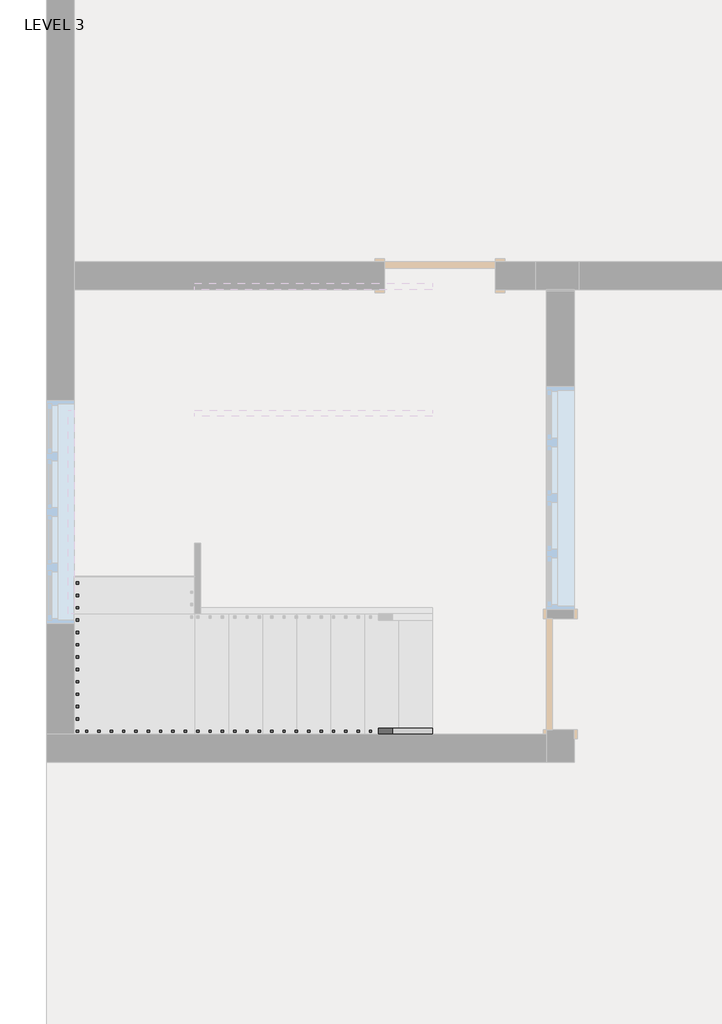
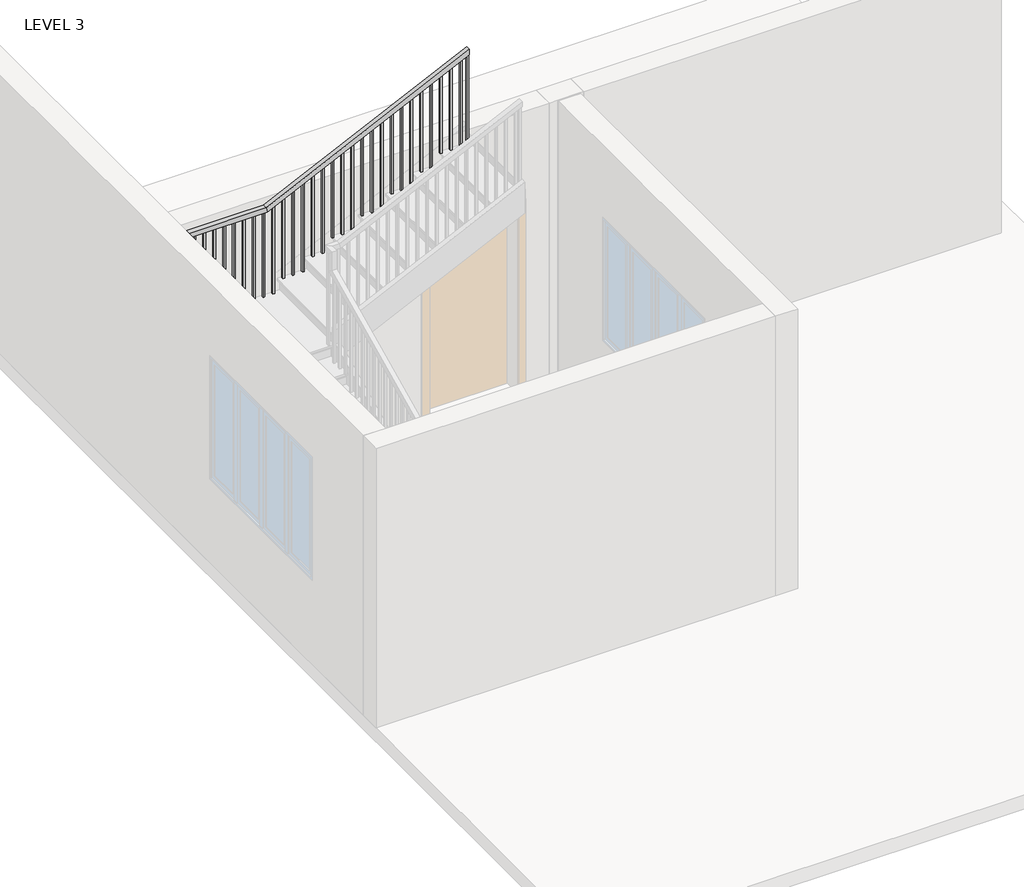
# One storey, part 2 of 3: 1 railing.
"""IFC4 building model written with IfcOpenShell, lengths in millimetres."""

from ifc_helpers import new_model, si_unit, frame, origin, place, context, project, spatial, polyline, outline, extrude, faceted_brep, element, save

model = new_model("IFC4")

# Units and contexts
model_context = context("Model", 3, world=origin())
ifc_project = project(units=[si_unit("LENGTHUNIT", "METRE", prefix="MILLI")], contexts=[model_context])

# Site, building, storey
site = spatial("IfcSite", under=ifc_project)
building = spatial("IfcBuilding", under=site)
storey = spatial("IfcBuildingStorey", under=building, Name="LEVEL 3", Elevation=6248.4)

# Railing
placement = place(None, origin())
element("IfcRailing", 1, ObjectType="Handrail - Rectangular", at=placement, inside=storey, context=model_context, shape_type="SolidModel", body=[
    faceted_brep([(-19769.8789184, -1118.4399287, 7295.3217391), (-19769.8789184, -1118.4399287, 7239.0971684), (-19769.8789184, -1067.6399287, 7239.0971684), (-19769.8789184, -1067.6399287, 7295.3217391), (-21865.3789184, -1118.4399287, 8289.2347826), (-21876.8157218, -1118.4399287, 8238.4347826), (-21876.8157218, -1067.6399287, 8238.4347826), (-21865.3789184, -1067.6399287, 8289.2347826), (-22716.2789184, -1118.4399287, 8238.4347826), (-22716.2789184, -1118.4399287, 8289.2347826), (-22716.2789184, -267.5399287, 8289.2347826), (-22716.2789184, -256.1031254, 8238.4347826), (-22665.4789184, -1067.6399287, 8238.4347826), (-22665.4789184, -256.1031254, 8238.4347826), (-22665.4789184, -1067.6399287, 8289.2347826), (-22665.4789184, -267.5399287, 8289.2347826), (-22716.2789184, 2539.1600713, 9166.0869565), (-22716.2789184, 2539.1600713, 9216.8869565), (-21865.3789184, 2539.1600713, 9216.8869565), (-21853.9421151, 2539.1600713, 9166.0869565), (-22665.4789184, 2488.3600713, 9166.0869565), (-21853.9421151, 2488.3600713, 9166.0869565), (-22665.4789184, 2488.3600713, 9216.8869565), (-21865.3789184, 2488.3600713, 9216.8869565), (-22716.2789184, 1688.2600713, 9216.8869565), (-22716.2789184, 1699.6968746, 9166.0869565), (-22665.4789184, 1699.6968746, 9166.0869565), (-22665.4789184, 1688.2600713, 9216.8869565), (-19769.8789184, 2539.1600713, 10210.8), (-19769.8789184, 2488.3600713, 10210.8), (-19769.8789184, 2488.3600713, 10154.5754292), (-19769.8789184, 2539.1600713, 10154.5754292)], [[[0, 1, 2, 3]], [[1, 0, 4, 5]], [[2, 1, 5, 6]], [[3, 2, 6, 7]], [[0, 3, 7, 4]], [[8, 9, 10, 11]], [[12, 8, 11, 13]], [[14, 12, 13, 15]], [[9, 14, 15, 10]], [[16, 17, 18, 19]], [[20, 16, 19, 21]], [[22, 20, 21, 23]], [[17, 22, 23, 18]], [[5, 4, 9, 8]], [[6, 5, 8, 12]], [[7, 6, 12, 14]], [[4, 7, 14, 9]], [[11, 10, 24, 25]], [[13, 11, 25, 26]], [[15, 13, 26, 27]], [[10, 15, 27, 24]], [[25, 24, 17, 16]], [[26, 25, 16, 20]], [[27, 26, 20, 22]], [[24, 27, 22, 17]], [[28, 29, 30, 31]], [[19, 18, 28, 31]], [[21, 19, 31, 30]], [[23, 21, 30, 29]], [[18, 23, 29, 28]]]),
    extrude(outline(polyline([(10113.9153502, -19855.6039184), (9163.8782609, -19855.6039184), (9163.8782609, -19836.5539184), (10122.9509233, -19836.5539184), (10113.9153502, -19855.6039184)])), frame((0.0, 2504.2350713, 0.0), z_axis=(0.0, 1.0, 0.0), x_axis=(0.0, 0.0, 1.0)), (0.0, 0.0, 1.0), 19.05),
    extrude(outline(polyline([(10065.7256269, -19957.2039184), (9163.8782609, -19957.2039184), (9163.8782609, -19938.1539184), (10074.7612, -19938.1539184), (10065.7256269, -19957.2039184)])), frame((0.0, 2504.2350713, 0.0), z_axis=(0.0, 1.0, 0.0), x_axis=(0.0, 0.0, 1.0)), (0.0, 0.0, 1.0), 19.05),
    extrude(outline(polyline([(10017.5359035, -20058.8039184), (9163.8782609, -20058.8039184), (9163.8782609, -20039.7539184), (10026.5714767, -20039.7539184), (10017.5359035, -20058.8039184)])), frame((0.0, 2504.2350713, 0.0), z_axis=(0.0, 1.0, 0.0), x_axis=(0.0, 0.0, 1.0)), (0.0, 0.0, 1.0), 19.05),
    extrude(outline(polyline([(9969.3461802, -20160.4039184), (9031.3565217, -20160.4039184), (9031.3565217, -20141.3539184), (9978.3817533, -20141.3539184), (9969.3461802, -20160.4039184)])), frame((0.0, 2504.2350713, 0.0), z_axis=(0.0, 1.0, 0.0), x_axis=(0.0, 0.0, 1.0)), (0.0, 0.0, 1.0), 19.05),
    extrude(outline(polyline([(9921.1564569, -20262.0039184), (9031.3565217, -20262.0039184), (9031.3565217, -20242.9539184), (9930.19203, -20242.9539184), (9921.1564569, -20262.0039184)])), frame((0.0, 2504.2350713, 0.0), z_axis=(0.0, 1.0, 0.0), x_axis=(0.0, 0.0, 1.0)), (0.0, 0.0, 1.0), 19.05),
    extrude(outline(polyline([(9872.9667336, -20363.6039184), (8898.8347826, -20363.6039184), (8898.8347826, -20344.5539184), (9882.0023067, -20344.5539184), (9872.9667336, -20363.6039184)])), frame((0.0, 2504.2350713, 0.0), z_axis=(0.0, 1.0, 0.0), x_axis=(0.0, 0.0, 1.0)), (0.0, 0.0, 1.0), 19.05),
    extrude(outline(polyline([(9824.7770103, -20465.2039184), (8898.8347826, -20465.2039184), (8898.8347826, -20446.1539184), (9833.8125834, -20446.1539184), (9824.7770103, -20465.2039184)])), frame((0.0, 2504.2350713, 0.0), z_axis=(0.0, 1.0, 0.0), x_axis=(0.0, 0.0, 1.0)), (0.0, 0.0, 1.0), 19.05),
    extrude(outline(polyline([(9776.5872869, -20566.8039184), (8898.8347826, -20566.8039184), (8898.8347826, -20547.7539184), (9785.6228601, -20547.7539184), (9776.5872869, -20566.8039184)])), frame((0.0, 2504.2350713, 0.0), z_axis=(0.0, 1.0, 0.0), x_axis=(0.0, 0.0, 1.0)), (0.0, 0.0, 1.0), 19.05),
    extrude(outline(polyline([(9728.3975636, -20668.4039184), (8766.3130435, -20668.4039184), (8766.3130435, -20649.3539184), (9737.4331367, -20649.3539184), (9728.3975636, -20668.4039184)])), frame((0.0, 2504.2350713, 0.0), z_axis=(0.0, 1.0, 0.0), x_axis=(0.0, 0.0, 1.0)), (0.0, 0.0, 1.0), 19.05),
    extrude(outline(polyline([(9680.2078403, -20770.0039184), (8766.3130435, -20770.0039184), (8766.3130435, -20750.9539184), (9689.2434134, -20750.9539184), (9680.2078403, -20770.0039184)])), frame((0.0, 2504.2350713, 0.0), z_axis=(0.0, 1.0, 0.0), x_axis=(0.0, 0.0, 1.0)), (0.0, 0.0, 1.0), 19.05),
    extrude(outline(polyline([(9632.018117, -20871.6039184), (8766.3130435, -20871.6039184), (8766.3130435, -20852.5539184), (9641.0536901, -20852.5539184), (9632.018117, -20871.6039184)])), frame((0.0, 2504.2350713, 0.0), z_axis=(0.0, 1.0, 0.0), x_axis=(0.0, 0.0, 1.0)), (0.0, 0.0, 1.0), 19.05),
    extrude(outline(polyline([(9583.8283937, -20973.2039184), (8633.7913043, -20973.2039184), (8633.7913043, -20954.1539184), (9592.8639668, -20954.1539184), (9583.8283937, -20973.2039184)])), frame((0.0, 2504.2350713, 0.0), z_axis=(0.0, 1.0, 0.0), x_axis=(0.0, 0.0, 1.0)), (0.0, 0.0, 1.0), 19.05),
    extrude(outline(polyline([(9535.6386703, -21074.8039184), (8633.7913043, -21074.8039184), (8633.7913043, -21055.7539184), (9544.6742435, -21055.7539184), (9535.6386703, -21074.8039184)])), frame((0.0, 2504.2350713, 0.0), z_axis=(0.0, 1.0, 0.0), x_axis=(0.0, 0.0, 1.0)), (0.0, 0.0, 1.0), 19.05),
    extrude(outline(polyline([(9487.448947, -21176.4039184), (8633.7913043, -21176.4039184), (8633.7913043, -21157.3539184), (9496.4845201, -21157.3539184), (9487.448947, -21176.4039184)])), frame((0.0, 2504.2350713, 0.0), z_axis=(0.0, 1.0, 0.0), x_axis=(0.0, 0.0, 1.0)), (0.0, 0.0, 1.0), 19.05),
    extrude(outline(polyline([(9439.2592237, -21278.0039184), (8501.2695652, -21278.0039184), (8501.2695652, -21258.9539184), (9448.2947968, -21258.9539184), (9439.2592237, -21278.0039184)])), frame((0.0, 2504.2350713, 0.0), z_axis=(0.0, 1.0, 0.0), x_axis=(0.0, 0.0, 1.0)), (0.0, 0.0, 1.0), 19.05),
    extrude(outline(polyline([(9391.0695004, -21379.6039184), (8501.2695652, -21379.6039184), (8501.2695652, -21360.5539184), (9400.1050735, -21360.5539184), (9391.0695004, -21379.6039184)])), frame((0.0, 2504.2350713, 0.0), z_axis=(0.0, 1.0, 0.0), x_axis=(0.0, 0.0, 1.0)), (0.0, 0.0, 1.0), 19.05),
    extrude(outline(polyline([(9342.8797771, -21481.2039184), (8368.7478261, -21481.2039184), (8368.7478261, -21462.1539184), (9351.9153502, -21462.1539184), (9342.8797771, -21481.2039184)])), frame((0.0, 2504.2350713, 0.0), z_axis=(0.0, 1.0, 0.0), x_axis=(0.0, 0.0, 1.0)), (0.0, 0.0, 1.0), 19.05),
    extrude(outline(polyline([(9294.6900537, -21582.8039184), (8368.7478261, -21582.8039184), (8368.7478261, -21563.7539184), (9303.7256269, -21563.7539184), (9294.6900537, -21582.8039184)])), frame((0.0, 2504.2350713, 0.0), z_axis=(0.0, 1.0, 0.0), x_axis=(0.0, 0.0, 1.0)), (0.0, 0.0, 1.0), 19.05),
    extrude(outline(polyline([(9246.5003304, -21684.4039184), (8368.7478261, -21684.4039184), (8368.7478261, -21665.3539184), (9255.5359035, -21665.3539184), (9246.5003304, -21684.4039184)])), frame((0.0, 2504.2350713, 0.0), z_axis=(0.0, 1.0, 0.0), x_axis=(0.0, 0.0, 1.0)), (0.0, 0.0, 1.0), 19.05),
    extrude(outline(polyline([(9198.3106071, -21786.0039184), (8236.226087, -21786.0039184), (8236.226087, -21766.9539184), (9207.3461802, -21766.9539184), (9198.3106071, -21786.0039184)])), frame((0.0, 2504.2350713, 0.0), z_axis=(0.0, 1.0, 0.0), x_axis=(0.0, 0.0, 1.0)), (0.0, 0.0, 1.0), 19.05),
    extrude(outline(polyline([(-21887.6039184, 2523.2850713), (-21868.5539184, 2523.2850713), (-21868.5539184, 2504.2350713), (-21887.6039184, 2504.2350713), (-21887.6039184, 2523.2850713)])), frame((0.0, 0.0, 8236.226087), z_axis=(0.0, 0.0, 1.0), x_axis=(1.0, 0.0, 0.0)), (0.0, 0.0, 1.0), 929.8608696),
    extrude(outline(polyline([(-21989.2039184, 2523.2850713), (-21970.1539184, 2523.2850713), (-21970.1539184, 2504.2350713), (-21989.2039184, 2504.2350713), (-21989.2039184, 2523.2850713)])), frame((0.0, 0.0, 8236.226087), z_axis=(0.0, 0.0, 1.0), x_axis=(1.0, 0.0, 0.0)), (0.0, 0.0, 1.0), 929.8608696),
    extrude(outline(polyline([(-22090.8039184, 2523.2850713), (-22071.7539184, 2523.2850713), (-22071.7539184, 2504.2350713), (-22090.8039184, 2504.2350713), (-22090.8039184, 2523.2850713)])), frame((0.0, 0.0, 8236.226087), z_axis=(0.0, 0.0, 1.0), x_axis=(1.0, 0.0, 0.0)), (0.0, 0.0, 1.0), 929.8608696),
    extrude(outline(polyline([(-22192.4039184, 2523.2850713), (-22173.3539184, 2523.2850713), (-22173.3539184, 2504.2350713), (-22192.4039184, 2504.2350713), (-22192.4039184, 2523.2850713)])), frame((0.0, 0.0, 8236.226087), z_axis=(0.0, 0.0, 1.0), x_axis=(1.0, 0.0, 0.0)), (0.0, 0.0, 1.0), 929.8608696),
    extrude(outline(polyline([(-22294.0039184, 2523.2850713), (-22274.9539184, 2523.2850713), (-22274.9539184, 2504.2350713), (-22294.0039184, 2504.2350713), (-22294.0039184, 2523.2850713)])), frame((0.0, 0.0, 8236.226087), z_axis=(0.0, 0.0, 1.0), x_axis=(1.0, 0.0, 0.0)), (0.0, 0.0, 1.0), 929.8608696),
    extrude(outline(polyline([(-22395.6039184, 2523.2850713), (-22376.5539184, 2523.2850713), (-22376.5539184, 2504.2350713), (-22395.6039184, 2504.2350713), (-22395.6039184, 2523.2850713)])), frame((0.0, 0.0, 8236.226087), z_axis=(0.0, 0.0, 1.0), x_axis=(1.0, 0.0, 0.0)), (0.0, 0.0, 1.0), 929.8608696),
    extrude(outline(polyline([(-22497.2039184, 2523.2850713), (-22478.1539184, 2523.2850713), (-22478.1539184, 2504.2350713), (-22497.2039184, 2504.2350713), (-22497.2039184, 2523.2850713)])), frame((0.0, 0.0, 8236.226087), z_axis=(0.0, 0.0, 1.0), x_axis=(1.0, 0.0, 0.0)), (0.0, 0.0, 1.0), 929.8608696),
    extrude(outline(polyline([(-22598.8039184, 2523.2850713), (-22579.7539184, 2523.2850713), (-22579.7539184, 2504.2350713), (-22598.8039184, 2504.2350713), (-22598.8039184, 2523.2850713)])), frame((0.0, 0.0, 8236.226087), z_axis=(0.0, 0.0, 1.0), x_axis=(1.0, 0.0, 0.0)), (0.0, 0.0, 1.0), 929.8608696),
    extrude(outline(polyline([(-22700.4039184, 2453.4350713), (-22700.4039184, 2472.4850713), (-22681.3539184, 2472.4850713), (-22681.3539184, 2453.4350713), (-22700.4039184, 2453.4350713)])), frame((0.0, 0.0, 8236.226087), z_axis=(0.0, 0.0, 1.0), x_axis=(1.0, 0.0, 0.0)), (0.0, 0.0, 1.0), 929.8608696),
    extrude(outline(polyline([(-22700.4039184, 2351.8350713), (-22700.4039184, 2370.8850713), (-22681.3539184, 2370.8850713), (-22681.3539184, 2351.8350713), (-22700.4039184, 2351.8350713)])), frame((0.0, 0.0, 8236.226087), z_axis=(0.0, 0.0, 1.0), x_axis=(1.0, 0.0, 0.0)), (0.0, 0.0, 1.0), 929.8608696),
    extrude(outline(polyline([(-22700.4039184, 2250.2350713), (-22700.4039184, 2269.2850713), (-22681.3539184, 2269.2850713), (-22681.3539184, 2250.2350713), (-22700.4039184, 2250.2350713)])), frame((0.0, 0.0, 8236.226087), z_axis=(0.0, 0.0, 1.0), x_axis=(1.0, 0.0, 0.0)), (0.0, 0.0, 1.0), 929.8608696),
    extrude(outline(polyline([(-22700.4039184, 2148.6350713), (-22700.4039184, 2167.6850713), (-22681.3539184, 2167.6850713), (-22681.3539184, 2148.6350713), (-22700.4039184, 2148.6350713)])), frame((0.0, 0.0, 8236.226087), z_axis=(0.0, 0.0, 1.0), x_axis=(1.0, 0.0, 0.0)), (0.0, 0.0, 1.0), 929.8608696),
    extrude(outline(polyline([(-22700.4039184, 2047.0350713), (-22700.4039184, 2066.0850713), (-22681.3539184, 2066.0850713), (-22681.3539184, 2047.0350713), (-22700.4039184, 2047.0350713)])), frame((0.0, 0.0, 8236.226087), z_axis=(0.0, 0.0, 1.0), x_axis=(1.0, 0.0, 0.0)), (0.0, 0.0, 1.0), 929.8608696),
    extrude(outline(polyline([(-22700.4039184, 1945.4350713), (-22700.4039184, 1964.4850713), (-22681.3539184, 1964.4850713), (-22681.3539184, 1945.4350713), (-22700.4039184, 1945.4350713)])), frame((0.0, 0.0, 8236.226087), z_axis=(0.0, 0.0, 1.0), x_axis=(1.0, 0.0, 0.0)), (0.0, 0.0, 1.0), 929.8608696),
    extrude(outline(polyline([(-22700.4039184, 1843.8350713), (-22700.4039184, 1862.8850713), (-22681.3539184, 1862.8850713), (-22681.3539184, 1843.8350713), (-22700.4039184, 1843.8350713)])), frame((0.0, 0.0, 8236.226087), z_axis=(0.0, 0.0, 1.0), x_axis=(1.0, 0.0, 0.0)), (0.0, 0.0, 1.0), 929.8608696),
    extrude(outline(polyline([(-22700.4039184, 1742.2350713), (-22700.4039184, 1761.2850713), (-22681.3539184, 1761.2850713), (-22681.3539184, 1742.2350713), (-22700.4039184, 1742.2350713)])), frame((0.0, 0.0, 8236.226087), z_axis=(0.0, 0.0, 1.0), x_axis=(1.0, 0.0, 0.0)), (0.0, 0.0, 1.0), 929.8608696),
    extrude(outline(polyline([(1659.6850713, 9147.1090261), (1659.6850713, 8236.226087), (1640.6350713, 8236.226087), (1640.6350713, 9138.0734529), (1659.6850713, 9147.1090261)])), frame((-22700.4039184, 0.0, 0.0), z_axis=(1.0, 0.0, 0.0), x_axis=(0.0, 1.0, 0.0)), (0.0, 0.0, 1.0), 19.05),
    extrude(outline(polyline([(1558.0850713, 9098.9193027), (1558.0850713, 8236.226087), (1539.0350713, 8236.226087), (1539.0350713, 9089.8837296), (1558.0850713, 9098.9193027)])), frame((-22700.4039184, 0.0, 0.0), z_axis=(1.0, 0.0, 0.0), x_axis=(0.0, 1.0, 0.0)), (0.0, 0.0, 1.0), 19.05),
    extrude(outline(polyline([(1456.4850713, 9050.7295794), (1456.4850713, 8103.7043478), (1437.4350713, 8103.7043478), (1437.4350713, 9041.6940063), (1456.4850713, 9050.7295794)])), frame((-22700.4039184, 0.0, 0.0), z_axis=(1.0, 0.0, 0.0), x_axis=(0.0, 1.0, 0.0)), (0.0, 0.0, 1.0), 19.05),
    extrude(outline(polyline([(1354.8850713, 9002.5398561), (1354.8850713, 8103.7043478), (1335.8350713, 8103.7043478), (1335.8350713, 8993.504283), (1354.8850713, 9002.5398561)])), frame((-22700.4039184, 0.0, 0.0), z_axis=(1.0, 0.0, 0.0), x_axis=(0.0, 1.0, 0.0)), (0.0, 0.0, 1.0), 19.05),
    extrude(outline(polyline([(1253.2850713, 8954.3501328), (1253.2850713, 7971.1826087), (1234.2350713, 7971.1826087), (1234.2350713, 8945.3145597), (1253.2850713, 8954.3501328)])), frame((-22700.4039184, 0.0, 0.0), z_axis=(1.0, 0.0, 0.0), x_axis=(0.0, 1.0, 0.0)), (0.0, 0.0, 1.0), 19.05),
    extrude(outline(polyline([(1151.6850713, 8906.1604095), (1151.6850713, 7971.1826087), (1132.6350713, 7971.1826087), (1132.6350713, 8897.1248363), (1151.6850713, 8906.1604095)])), frame((-22700.4039184, 0.0, 0.0), z_axis=(1.0, 0.0, 0.0), x_axis=(0.0, 1.0, 0.0)), (0.0, 0.0, 1.0), 19.05),
    extrude(outline(polyline([(1050.0850713, 8857.9706861), (1050.0850713, 7971.1826087), (1031.0350713, 7971.1826087), (1031.0350713, 8848.935113), (1050.0850713, 8857.9706861)])), frame((-22700.4039184, 0.0, 0.0), z_axis=(1.0, 0.0, 0.0), x_axis=(0.0, 1.0, 0.0)), (0.0, 0.0, 1.0), 19.05),
    extrude(outline(polyline([(948.4850713, 8809.7809628), (948.4850713, 7838.6608696), (929.4350713, 7838.6608696), (929.4350713, 8800.7453897), (948.4850713, 8809.7809628)])), frame((-22700.4039184, 0.0, 0.0), z_axis=(1.0, 0.0, 0.0), x_axis=(0.0, 1.0, 0.0)), (0.0, 0.0, 1.0), 19.05),
    extrude(outline(polyline([(846.8850713, 8761.5912395), (846.8850713, 7838.6608696), (827.8350713, 7838.6608696), (827.8350713, 8752.5556664), (846.8850713, 8761.5912395)])), frame((-22700.4039184, 0.0, 0.0), z_axis=(1.0, 0.0, 0.0), x_axis=(0.0, 1.0, 0.0)), (0.0, 0.0, 1.0), 19.05),
    extrude(outline(polyline([(745.2850713, 8713.4015162), (745.2850713, 7838.6608696), (726.2350713, 7838.6608696), (726.2350713, 8704.3659431), (745.2850713, 8713.4015162)])), frame((-22700.4039184, 0.0, 0.0), z_axis=(1.0, 0.0, 0.0), x_axis=(0.0, 1.0, 0.0)), (0.0, 0.0, 1.0), 19.05),
    extrude(outline(polyline([(643.6850713, 8665.2117929), (643.6850713, 7706.1391304), (624.6350713, 7706.1391304), (624.6350713, 8656.1762197), (643.6850713, 8665.2117929)])), frame((-22700.4039184, 0.0, 0.0), z_axis=(1.0, 0.0, 0.0), x_axis=(0.0, 1.0, 0.0)), (0.0, 0.0, 1.0), 19.05),
    extrude(outline(polyline([(542.0850713, 8617.0220695), (542.0850713, 7706.1391304), (523.0350713, 7706.1391304), (523.0350713, 8607.9864964), (542.0850713, 8617.0220695)])), frame((-22700.4039184, 0.0, 0.0), z_axis=(1.0, 0.0, 0.0), x_axis=(0.0, 1.0, 0.0)), (0.0, 0.0, 1.0), 19.05),
    extrude(outline(polyline([(440.4850713, 8568.8323462), (440.4850713, 7706.1391304), (421.4350713, 7706.1391304), (421.4350713, 8559.7967731), (440.4850713, 8568.8323462)])), frame((-22700.4039184, 0.0, 0.0), z_axis=(1.0, 0.0, 0.0), x_axis=(0.0, 1.0, 0.0)), (0.0, 0.0, 1.0), 19.05),
    extrude(outline(polyline([(338.8850713, 8520.6426229), (338.8850713, 7573.6173913), (319.8350713, 7573.6173913), (319.8350713, 8511.6070498), (338.8850713, 8520.6426229)])), frame((-22700.4039184, 0.0, 0.0), z_axis=(1.0, 0.0, 0.0), x_axis=(0.0, 1.0, 0.0)), (0.0, 0.0, 1.0), 19.05),
    extrude(outline(polyline([(237.2850713, 8472.4528996), (237.2850713, 7573.6173913), (218.2350713, 7573.6173913), (218.2350713, 8463.4173265), (237.2850713, 8472.4528996)])), frame((-22700.4039184, 0.0, 0.0), z_axis=(1.0, 0.0, 0.0), x_axis=(0.0, 1.0, 0.0)), (0.0, 0.0, 1.0), 19.05),
    extrude(outline(polyline([(135.6850713, 8424.2631763), (135.6850713, 7441.0956522), (116.6350713, 7441.0956522), (116.6350713, 8415.2276031), (135.6850713, 8424.2631763)])), frame((-22700.4039184, 0.0, 0.0), z_axis=(1.0, 0.0, 0.0), x_axis=(0.0, 1.0, 0.0)), (0.0, 0.0, 1.0), 19.05),
    extrude(outline(polyline([(34.0850713, 8376.0734529), (34.0850713, 7441.0956522), (15.0350713, 7441.0956522), (15.0350713, 8367.0378798), (34.0850713, 8376.0734529)])), frame((-22700.4039184, 0.0, 0.0), z_axis=(1.0, 0.0, 0.0), x_axis=(0.0, 1.0, 0.0)), (0.0, 0.0, 1.0), 19.05),
    extrude(outline(polyline([(-67.5149287, 8327.8837296), (-67.5149287, 7441.0956522), (-86.5649287, 7441.0956522), (-86.5649287, 8318.8481565), (-67.5149287, 8327.8837296)])), frame((-22700.4039184, 0.0, 0.0), z_axis=(1.0, 0.0, 0.0), x_axis=(0.0, 1.0, 0.0)), (0.0, 0.0, 1.0), 19.05),
    extrude(outline(polyline([(-169.1149287, 8279.6940063), (-169.1149287, 7308.573913), (-188.1649287, 7308.573913), (-188.1649287, 8270.6584332), (-169.1149287, 8279.6940063)])), frame((-22700.4039184, 0.0, 0.0), z_axis=(1.0, 0.0, 0.0), x_axis=(0.0, 1.0, 0.0)), (0.0, 0.0, 1.0), 19.05),
    extrude(outline(polyline([(-22700.4039184, -289.7649287), (-22700.4039184, -270.7149287), (-22681.3539184, -270.7149287), (-22681.3539184, -289.7649287), (-22700.4039184, -289.7649287)])), frame((0.0, 0.0, 7308.573913), z_axis=(0.0, 0.0, 1.0), x_axis=(1.0, 0.0, 0.0)), (0.0, 0.0, 1.0), 929.8608696),
    extrude(outline(polyline([(-22700.4039184, -391.3649287), (-22700.4039184, -372.3149287), (-22681.3539184, -372.3149287), (-22681.3539184, -391.3649287), (-22700.4039184, -391.3649287)])), frame((0.0, 0.0, 7308.573913), z_axis=(0.0, 0.0, 1.0), x_axis=(1.0, 0.0, 0.0)), (0.0, 0.0, 1.0), 929.8608696),
    extrude(outline(polyline([(-22700.4039184, -492.9649287), (-22700.4039184, -473.9149287), (-22681.3539184, -473.9149287), (-22681.3539184, -492.9649287), (-22700.4039184, -492.9649287)])), frame((0.0, 0.0, 7308.573913), z_axis=(0.0, 0.0, 1.0), x_axis=(1.0, 0.0, 0.0)), (0.0, 0.0, 1.0), 929.8608696),
    extrude(outline(polyline([(-22700.4039184, -594.5649287), (-22700.4039184, -575.5149287), (-22681.3539184, -575.5149287), (-22681.3539184, -594.5649287), (-22700.4039184, -594.5649287)])), frame((0.0, 0.0, 7308.573913), z_axis=(0.0, 0.0, 1.0), x_axis=(1.0, 0.0, 0.0)), (0.0, 0.0, 1.0), 929.8608696),
    extrude(outline(polyline([(-22700.4039184, -696.1649287), (-22700.4039184, -677.1149287), (-22681.3539184, -677.1149287), (-22681.3539184, -696.1649287), (-22700.4039184, -696.1649287)])), frame((0.0, 0.0, 7308.573913), z_axis=(0.0, 0.0, 1.0), x_axis=(1.0, 0.0, 0.0)), (0.0, 0.0, 1.0), 929.8608696),
    extrude(outline(polyline([(-22700.4039184, -797.7649287), (-22700.4039184, -778.7149287), (-22681.3539184, -778.7149287), (-22681.3539184, -797.7649287), (-22700.4039184, -797.7649287)])), frame((0.0, 0.0, 7308.573913), z_axis=(0.0, 0.0, 1.0), x_axis=(1.0, 0.0, 0.0)), (0.0, 0.0, 1.0), 929.8608696),
    extrude(outline(polyline([(-22700.4039184, -899.3649287), (-22700.4039184, -880.3149287), (-22681.3539184, -880.3149287), (-22681.3539184, -899.3649287), (-22700.4039184, -899.3649287)])), frame((0.0, 0.0, 7308.573913), z_axis=(0.0, 0.0, 1.0), x_axis=(1.0, 0.0, 0.0)), (0.0, 0.0, 1.0), 929.8608696),
    extrude(outline(polyline([(-22700.4039184, -1000.9649287), (-22700.4039184, -981.9149287), (-22681.3539184, -981.9149287), (-22681.3539184, -1000.9649287), (-22700.4039184, -1000.9649287)])), frame((0.0, 0.0, 7308.573913), z_axis=(0.0, 0.0, 1.0), x_axis=(1.0, 0.0, 0.0)), (0.0, 0.0, 1.0), 929.8608696),
    extrude(outline(polyline([(-22605.1539184, -1102.5649287), (-22624.2039184, -1102.5649287), (-22624.2039184, -1083.5149287), (-22605.1539184, -1083.5149287), (-22605.1539184, -1102.5649287)])), frame((0.0, 0.0, 7308.573913), z_axis=(0.0, 0.0, 1.0), x_axis=(1.0, 0.0, 0.0)), (0.0, 0.0, 1.0), 929.8608696),
    extrude(outline(polyline([(-22503.5539184, -1102.5649287), (-22522.6039184, -1102.5649287), (-22522.6039184, -1083.5149287), (-22503.5539184, -1083.5149287), (-22503.5539184, -1102.5649287)])), frame((0.0, 0.0, 7308.573913), z_axis=(0.0, 0.0, 1.0), x_axis=(1.0, 0.0, 0.0)), (0.0, 0.0, 1.0), 929.8608696),
    extrude(outline(polyline([(-22401.9539184, -1102.5649287), (-22421.0039184, -1102.5649287), (-22421.0039184, -1083.5149287), (-22401.9539184, -1083.5149287), (-22401.9539184, -1102.5649287)])), frame((0.0, 0.0, 7308.573913), z_axis=(0.0, 0.0, 1.0), x_axis=(1.0, 0.0, 0.0)), (0.0, 0.0, 1.0), 929.8608696),
    extrude(outline(polyline([(-22300.3539184, -1102.5649287), (-22319.4039184, -1102.5649287), (-22319.4039184, -1083.5149287), (-22300.3539184, -1083.5149287), (-22300.3539184, -1102.5649287)])), frame((0.0, 0.0, 7308.573913), z_axis=(0.0, 0.0, 1.0), x_axis=(1.0, 0.0, 0.0)), (0.0, 0.0, 1.0), 929.8608696),
    extrude(outline(polyline([(-22198.7539184, -1102.5649287), (-22217.8039184, -1102.5649287), (-22217.8039184, -1083.5149287), (-22198.7539184, -1083.5149287), (-22198.7539184, -1102.5649287)])), frame((0.0, 0.0, 7308.573913), z_axis=(0.0, 0.0, 1.0), x_axis=(1.0, 0.0, 0.0)), (0.0, 0.0, 1.0), 929.8608696),
    extrude(outline(polyline([(-22097.1539184, -1102.5649287), (-22116.2039184, -1102.5649287), (-22116.2039184, -1083.5149287), (-22097.1539184, -1083.5149287), (-22097.1539184, -1102.5649287)])), frame((0.0, 0.0, 7308.573913), z_axis=(0.0, 0.0, 1.0), x_axis=(1.0, 0.0, 0.0)), (0.0, 0.0, 1.0), 929.8608696),
    extrude(outline(polyline([(-21995.5539184, -1102.5649287), (-22014.6039184, -1102.5649287), (-22014.6039184, -1083.5149287), (-21995.5539184, -1083.5149287), (-21995.5539184, -1102.5649287)])), frame((0.0, 0.0, 7308.573913), z_axis=(0.0, 0.0, 1.0), x_axis=(1.0, 0.0, 0.0)), (0.0, 0.0, 1.0), 929.8608696),
    extrude(outline(polyline([(-21893.9539184, -1102.5649287), (-21913.0039184, -1102.5649287), (-21913.0039184, -1083.5149287), (-21893.9539184, -1083.5149287), (-21893.9539184, -1102.5649287)])), frame((0.0, 0.0, 7308.573913), z_axis=(0.0, 0.0, 1.0), x_axis=(1.0, 0.0, 0.0)), (0.0, 0.0, 1.0), 929.8608696),
    extrude(outline(polyline([(8207.4094213, -21811.4039184), (7308.573913, -21811.4039184), (7308.573913, -21792.3539184), (8198.3738482, -21792.3539184), (8207.4094213, -21811.4039184)])), frame((0.0, -1102.5649287, 0.0), z_axis=(0.0, 1.0, 0.0), x_axis=(0.0, 0.0, 1.0)), (0.0, 0.0, 1.0), 19.05),
    extrude(outline(polyline([(8159.219698, -21709.8039184), (7176.0521739, -21709.8039184), (7176.0521739, -21690.7539184), (8150.1841249, -21690.7539184), (8159.219698, -21709.8039184)])), frame((0.0, -1102.5649287, 0.0), z_axis=(0.0, 1.0, 0.0), x_axis=(0.0, 0.0, 1.0)), (0.0, 0.0, 1.0), 19.05),
    extrude(outline(polyline([(8111.0299747, -21608.2039184), (7176.0521739, -21608.2039184), (7176.0521739, -21589.1539184), (8101.9944016, -21589.1539184), (8111.0299747, -21608.2039184)])), frame((0.0, -1102.5649287, 0.0), z_axis=(0.0, 1.0, 0.0), x_axis=(0.0, 0.0, 1.0)), (0.0, 0.0, 1.0), 19.05),
    extrude(outline(polyline([(8062.8402514, -21506.6039184), (7176.0521739, -21506.6039184), (7176.0521739, -21487.5539184), (8053.8046782, -21487.5539184), (8062.8402514, -21506.6039184)])), frame((0.0, -1102.5649287, 0.0), z_axis=(0.0, 1.0, 0.0), x_axis=(0.0, 0.0, 1.0)), (0.0, 0.0, 1.0), 19.05),
    extrude(outline(polyline([(8014.650528, -21405.0039184), (7043.5304348, -21405.0039184), (7043.5304348, -21385.9539184), (8005.6149549, -21385.9539184), (8014.650528, -21405.0039184)])), frame((0.0, -1102.5649287, 0.0), z_axis=(0.0, 1.0, 0.0), x_axis=(0.0, 0.0, 1.0)), (0.0, 0.0, 1.0), 19.05),
    extrude(outline(polyline([(7966.4608047, -21303.4039184), (7043.5304348, -21303.4039184), (7043.5304348, -21284.3539184), (7957.4252316, -21284.3539184), (7966.4608047, -21303.4039184)])), frame((0.0, -1102.5649287, 0.0), z_axis=(0.0, 1.0, 0.0), x_axis=(0.0, 0.0, 1.0)), (0.0, 0.0, 1.0), 19.05),
    extrude(outline(polyline([(7918.2710814, -21201.8039184), (7043.5304348, -21201.8039184), (7043.5304348, -21182.7539184), (7909.2355083, -21182.7539184), (7918.2710814, -21201.8039184)])), frame((0.0, -1102.5649287, 0.0), z_axis=(0.0, 1.0, 0.0), x_axis=(0.0, 0.0, 1.0)), (0.0, 0.0, 1.0), 19.05),
    extrude(outline(polyline([(7870.0813581, -21100.2039184), (6911.0086957, -21100.2039184), (6911.0086957, -21081.1539184), (7861.045785, -21081.1539184), (7870.0813581, -21100.2039184)])), frame((0.0, -1102.5649287, 0.0), z_axis=(0.0, 1.0, 0.0), x_axis=(0.0, 0.0, 1.0)), (0.0, 0.0, 1.0), 19.05),
    extrude(outline(polyline([(7821.8916348, -20998.6039184), (6911.0086957, -20998.6039184), (6911.0086957, -20979.5539184), (7812.8560616, -20979.5539184), (7821.8916348, -20998.6039184)])), frame((0.0, -1102.5649287, 0.0), z_axis=(0.0, 1.0, 0.0), x_axis=(0.0, 0.0, 1.0)), (0.0, 0.0, 1.0), 19.05),
    extrude(outline(polyline([(7773.7019114, -20897.0039184), (6911.0086957, -20897.0039184), (6911.0086957, -20877.9539184), (7764.6663383, -20877.9539184), (7773.7019114, -20897.0039184)])), frame((0.0, -1102.5649287, 0.0), z_axis=(0.0, 1.0, 0.0), x_axis=(0.0, 0.0, 1.0)), (0.0, 0.0, 1.0), 19.05),
    extrude(outline(polyline([(7725.5121881, -20795.4039184), (6778.4869565, -20795.4039184), (6778.4869565, -20776.3539184), (7716.476615, -20776.3539184), (7725.5121881, -20795.4039184)])), frame((0.0, -1102.5649287, 0.0), z_axis=(0.0, 1.0, 0.0), x_axis=(0.0, 0.0, 1.0)), (0.0, 0.0, 1.0), 19.05),
    extrude(outline(polyline([(7677.3224648, -20693.8039184), (6778.4869565, -20693.8039184), (6778.4869565, -20674.7539184), (7668.2868917, -20674.7539184), (7677.3224648, -20693.8039184)])), frame((0.0, -1102.5649287, 0.0), z_axis=(0.0, 1.0, 0.0), x_axis=(0.0, 0.0, 1.0)), (0.0, 0.0, 1.0), 19.05),
    extrude(outline(polyline([(7629.1327415, -20592.2039184), (6645.9652174, -20592.2039184), (6645.9652174, -20573.1539184), (7620.0971684, -20573.1539184), (7629.1327415, -20592.2039184)])), frame((0.0, -1102.5649287, 0.0), z_axis=(0.0, 1.0, 0.0), x_axis=(0.0, 0.0, 1.0)), (0.0, 0.0, 1.0), 19.05),
    extrude(outline(polyline([(7580.9430182, -20490.6039184), (6645.9652174, -20490.6039184), (6645.9652174, -20471.5539184), (7571.907445, -20471.5539184), (7580.9430182, -20490.6039184)])), frame((0.0, -1102.5649287, 0.0), z_axis=(0.0, 1.0, 0.0), x_axis=(0.0, 0.0, 1.0)), (0.0, 0.0, 1.0), 19.05),
    extrude(outline(polyline([(7532.7532948, -20389.0039184), (6645.9652174, -20389.0039184), (6645.9652174, -20369.9539184), (7523.7177217, -20369.9539184), (7532.7532948, -20389.0039184)])), frame((0.0, -1102.5649287, 0.0), z_axis=(0.0, 1.0, 0.0), x_axis=(0.0, 0.0, 1.0)), (0.0, 0.0, 1.0), 19.05),
    extrude(outline(polyline([(7484.5635715, -20287.4039184), (6513.4434783, -20287.4039184), (6513.4434783, -20268.3539184), (7475.5279984, -20268.3539184), (7484.5635715, -20287.4039184)])), frame((0.0, -1102.5649287, 0.0), z_axis=(0.0, 1.0, 0.0), x_axis=(0.0, 0.0, 1.0)), (0.0, 0.0, 1.0), 19.05),
    extrude(outline(polyline([(7436.3738482, -20185.8039184), (6513.4434783, -20185.8039184), (6513.4434783, -20166.7539184), (7427.3382751, -20166.7539184), (7436.3738482, -20185.8039184)])), frame((0.0, -1102.5649287, 0.0), z_axis=(0.0, 1.0, 0.0), x_axis=(0.0, 0.0, 1.0)), (0.0, 0.0, 1.0), 19.05),
    extrude(outline(polyline([(7388.1841249, -20084.2039184), (6513.4434783, -20084.2039184), (6513.4434783, -20065.1539184), (7379.1485518, -20065.1539184), (7388.1841249, -20084.2039184)])), frame((0.0, -1102.5649287, 0.0), z_axis=(0.0, 1.0, 0.0), x_axis=(0.0, 0.0, 1.0)), (0.0, 0.0, 1.0), 19.05),
    extrude(outline(polyline([(7339.9944016, -19982.6039184), (6380.9217391, -19982.6039184), (6380.9217391, -19963.5539184), (7330.9588284, -19963.5539184), (7339.9944016, -19982.6039184)])), frame((0.0, -1102.5649287, 0.0), z_axis=(0.0, 1.0, 0.0), x_axis=(0.0, 0.0, 1.0)), (0.0, 0.0, 1.0), 19.05),
    extrude(outline(polyline([(7291.8046782, -19881.0039184), (6380.9217391, -19881.0039184), (6380.9217391, -19861.9539184), (7282.7691051, -19861.9539184), (7291.8046782, -19881.0039184)])), frame((0.0, -1102.5649287, 0.0), z_axis=(0.0, 1.0, 0.0), x_axis=(0.0, 0.0, 1.0)), (0.0, 0.0, 1.0), 19.05),
    extrude(outline(polyline([(-22700.4039184, 2504.2350713), (-22700.4039184, 2523.2850713), (-22681.3539184, 2523.2850713), (-22681.3539184, 2504.2350713), (-22700.4039184, 2504.2350713)])), frame((0.0, 0.0, 8236.226087), z_axis=(0.0, 0.0, 1.0), x_axis=(1.0, 0.0, 0.0)), (0.0, 0.0, 1.0), 929.8608696),
    extrude(outline(polyline([(-22681.3539184, -1102.5649287), (-22700.4039184, -1102.5649287), (-22700.4039184, -1083.5149287), (-22681.3539184, -1083.5149287), (-22681.3539184, -1102.5649287)])), frame((0.0, 0.0, 7308.573913), z_axis=(0.0, 0.0, 1.0), x_axis=(1.0, 0.0, 0.0)), (0.0, 0.0, 1.0), 929.8608696),
    extrude(outline(polyline([(10145.5398561, -19788.9289184), (9163.8782609, -19788.9289184), (9163.8782609, -19769.8789184), (10154.5754292, -19769.8789184), (10145.5398561, -19788.9289184)])), frame((0.0, 2504.2350713, 0.0), z_axis=(0.0, 1.0, 0.0), x_axis=(0.0, 0.0, 1.0)), (0.0, 0.0, 1.0), 19.05),
    extrude(outline(polyline([(7248.1327415, -19788.9289184), (6380.9217391, -19788.9289184), (6380.9217391, -19769.8789184), (7239.0971684, -19769.8789184), (7248.1327415, -19788.9289184)])), frame((0.0, -1102.5649287, 0.0), z_axis=(0.0, 1.0, 0.0), x_axis=(0.0, 0.0, 1.0)), (0.0, 0.0, 1.0), 19.05),
])

save(model, "model.ifc")

# Revit data of these elements
# Type "Handrail - Rectangular"
#   Assembly Code = "C2010400"
#   built-in parameter 1008612 = 0.0416667 (stored number, unit not read)
#   built-in parameter 1008611 = 0.0416667 (stored number, unit not read)
#   built-in parameter 1008609 = 0.333333 (stored number, unit not read)
#   built-in parameter 1008604 = 0.166667 (stored number, unit not read)
#   built-in parameter 1008603 = 0.166667 (stored number, unit not read)
#   Railing Height = 3' - 0"
#   built-in parameter 1008630 = 2
#   built-in parameter 1008610 = 2
#   built-in parameter 1008618 = Baluster - Square : 3/4"
# Element 1 (IfcRailing, "Handrail - Rectangular")
#   Phase Created = New Construction
#   Materials on its faces: "Wood - Birch - Solid Stained Light Low Gloss", "1 wall"
# Materials
#   "Wood - Birch - Solid Stained Light Low Gloss": class "Wood", colour RGB 210 159 95, transparency 0, Cost = 0
#   "1 wall": class "Glass", colour RGB 0 0 255, transparency 0.75, Cost = 0
